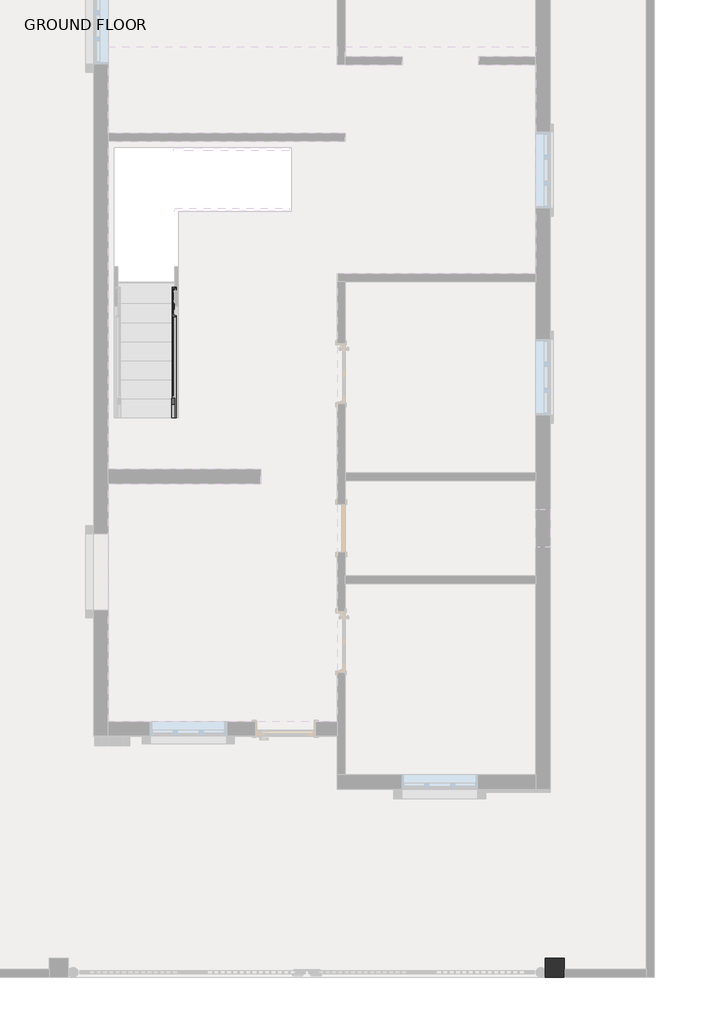
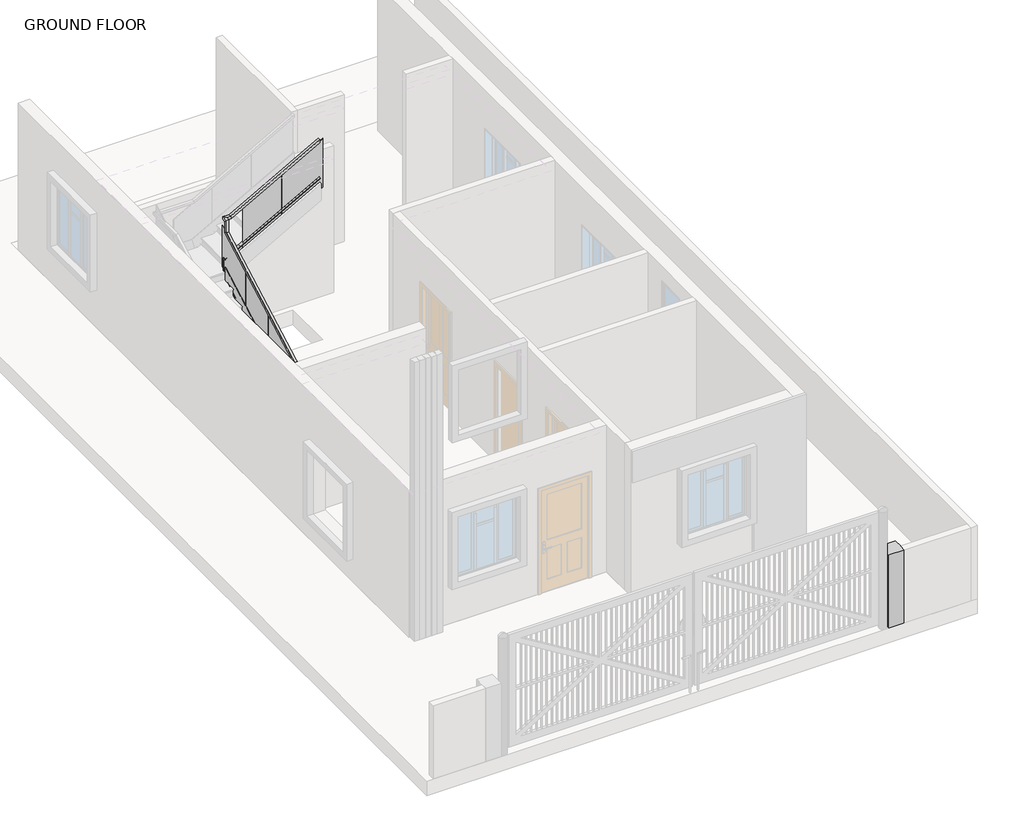
# One storey, part 2 of 4: 1 column, 1 railing.
"""IFC4 building model written with IfcOpenShell, lengths in millimetres."""

from ifc_helpers import new_model, si_unit, frame, origin, place, context, project, spatial, polyline, ellipse_curve, outline, extrude, faceted_brep, element, save
from ifc_brep_helpers import plane_surface, cylinder_surface, revolved_surface, advanced_brep

model = new_model("IFC4")

# Units and contexts
model_context = context("Model", 3, world=origin())
ifc_project = project(units=[si_unit("LENGTHUNIT", "METRE", prefix="MILLI")], contexts=[model_context])

# Site, building, storey
site = spatial("IfcSite", under=ifc_project)
building = spatial("IfcBuilding", under=site)
storey = spatial("IfcBuildingStorey", under=building, Name="GROUND FLOOR", Elevation=304.8)

# Column
placement = place(None, origin())
element("IfcColumn", 1, ObjectType="Rectangular Column : 1'X 1'", at=placement, inside=storey, context=model_context, shape_type="Brep", body=[
    faceted_brep([(-2180.0610805, -9269.5210084, 304.8), (-2180.0610805, -9447.3210084, 304.8), (-2180.0610805, -9574.3210084, 304.8), (-2484.8610805, -9574.3210084, 304.8), (-2484.8610805, -9269.5210084, 304.8), (-2180.0610805, -9269.5210084, 1828.8), (-2180.0610805, -9447.3210084, 1828.8), (-2180.0610805, -9574.3210084, 1828.8), (-2484.8610805, -9574.3210084, 1828.8), (-2484.8610805, -9269.5210084, 1828.8)], [[[0, 1, 2, 3, 4]], [[5, 6, 7, 2, 1, 0]], [[7, 8, 3, 2]], [[8, 9, 4, 3]], [[9, 5, 0, 4]], [[5, 9, 8, 7, 6]]]),
])

# Railing
element("IfcRailing", 2, ObjectType="GLASS PANEL RAILING", at=placement, inside=storey, context=model_context, shape_type="SolidModel", body=[
    faceted_brep([(-8451.9607439, -642.5827462, 1388.5333333), (-8451.9607439, -642.5827462, 1330.420221), (-8401.1607439, -642.5827462, 1330.420221), (-8401.1607439, -642.5827462, 1388.5333333), (-8451.9607439, 2634.0172538, 3208.8666667), (-8451.9607439, 2684.8172538, 3178.9757765), (-8401.1607439, 2684.8172538, 3178.9757765), (-8401.1607439, 2634.0172538, 3208.8666667), (-8451.9607439, 2634.0172538, 3462.8666667), (-8451.9607439, 2684.8172538, 3412.0666667), (-8401.1607439, 2684.8172538, 3412.0666667), (-8401.1607439, 2634.0172538, 3462.8666667), (-8451.9607439, 2761.0172538, 3462.8666667), (-8451.9607439, 2761.0172538, 3412.0666667), (-8401.1607439, 2710.2172538, 3412.0666667), (-8401.1607439, 2710.2172538, 3462.8666667), (-8324.9607439, 2761.0172538, 3462.8666667), (-8311.7971417, 2761.0172538, 3412.0666667), (-8311.7971417, 2710.2172538, 3412.0666667), (-8324.9607439, 2710.2172538, 3462.8666667), (-6572.3607439, 2761.0172538, 4436.5333333), (-6572.3607439, 2710.2172538, 4436.5333333), (-6572.3607439, 2710.2172538, 4378.420221), (-6572.3607439, 2761.0172538, 4378.420221)], [[[0, 1, 2, 3]], [[1, 0, 4, 5]], [[2, 1, 5, 6]], [[3, 2, 6, 7]], [[0, 3, 7, 4]], [[5, 4, 8, 9]], [[6, 5, 9, 10]], [[7, 6, 10, 11]], [[4, 7, 11, 8]], [[9, 8, 12, 13]], [[10, 9, 13, 14]], [[11, 10, 14, 15]], [[8, 11, 15, 12]], [[13, 12, 16, 17]], [[14, 13, 17, 18]], [[15, 14, 18, 19]], [[12, 15, 19, 16]], [[20, 21, 22, 23]], [[17, 16, 20, 23]], [[18, 17, 23, 22]], [[19, 18, 22, 21]], [[16, 19, 21, 20]]]),
    advanced_brep(
    [(-8441.4451439, -642.5827462, 604.8878361), (-8441.4451439, -642.5827462, 343.3788305), (-8378.1991439, -642.5827462, 343.3788305), (-8378.1991439, -642.5827462, 344.957123), (-8382.5819531, -642.5827462, 350.8756626), (-8406.2026439, -642.5827462, 355.3791882), (-8425.4405255, -642.5827462, 359.0470866), (-8434.2061439, -642.5827462, 370.8841659), (-8434.2061439, -642.5827462, 577.3825008), (-8425.4405255, -642.5827462, 589.2195801), (-8406.2026439, -642.5827462, 592.8874784), (-8382.5819531, -642.5827462, 597.391004), (-8378.1991439, -642.5827462, 603.3095437), (-8378.1991439, -642.5827462, 604.8878361), (-8441.4451439, 2687.2556538, 2454.7980583), (-8378.1991439, 2687.2556538, 2454.7980583), (-8378.1991439, 2687.2556538, 2453.2197659), (-8382.5819531, 2687.2556538, 2447.3012262), (-8406.2026439, 2687.2556538, 2442.7977006), (-8425.4405255, 2687.2556538, 2439.1298023), (-8434.2061439, 2687.2556538, 2427.292723), (-8434.2061439, 2687.2556538, 2220.7943881), (-8425.4405255, 2687.2556538, 2208.9573088), (-8406.2026439, 2687.2556538, 2205.2894105), (-8382.5819531, 2687.2556538, 2200.7858849), (-8378.1991439, 2687.2556538, 2194.8673452), (-8378.1991439, 2687.2556538, 2193.2890528), (-8441.4451439, 2687.2556538, 2193.2890528)],
    [
        (0, 1),
        (1, 2),
        (2, 3),
        (3, 4, ellipse_curve(frame((-8383.4442439, -642.5827462, 344.957123), z_axis=(0.0, -1.0, 0.0), x_axis=(0.0, 0.0, -1.0)), 6.0001789, 5.2451)),
        (4, 5),
        (5, 6),
        (6, 7, ellipse_curve(frame((-8423.7159439, -642.5827462, 370.8841659), z_axis=(0.0, 1.0, 0.0), x_axis=(0.0, 0.0, 1.0)), 12.0003577, 10.4902)),
        (7, 8),
        (8, 9, ellipse_curve(frame((-8423.7159439, -642.5827462, 577.3825008), z_axis=(0.0, 1.0, 0.0), x_axis=(0.0, 0.0, 1.0)), 12.0003577, 10.4902)),
        (9, 10),
        (10, 11),
        (11, 12, ellipse_curve(frame((-8383.4442439, -642.5827462, 603.3095437), z_axis=(0.0, -1.0, 0.0), x_axis=(0.0, 0.0, -1.0)), 6.0001789, 5.2451)),
        (12, 13),
        (13, 0),
        (14, 15),
        (15, 16),
        (16, 17, ellipse_curve(frame((-8383.4442439, 2687.2556538, 2453.2197659), z_axis=(0.0, 1.0, 0.0), x_axis=(0.0, 0.0, -1.0)), 6.0001789, 5.2451)),
        (17, 18),
        (18, 19),
        (19, 20, ellipse_curve(frame((-8423.7159439, 2687.2556538, 2427.292723), z_axis=(0.0, -1.0, 0.0), x_axis=(0.0, 0.0, 1.0)), 12.0003577, 10.4902)),
        (20, 21),
        (21, 22, ellipse_curve(frame((-8423.7159439, 2687.2556538, 2220.7943881), z_axis=(0.0, -1.0, 0.0), x_axis=(0.0, 0.0, 1.0)), 12.0003577, 10.4902)),
        (22, 23),
        (23, 24),
        (24, 25, ellipse_curve(frame((-8383.4442439, 2687.2556538, 2194.8673452), z_axis=(0.0, 1.0, 0.0), x_axis=(0.0, 0.0, -1.0)), 6.0001789, 5.2451)),
        (25, 26),
        (26, 27),
        (27, 14),
        (0, 14),
        (27, 1),
        (26, 2),
        (25, 3),
        (24, 4),
        (23, 5),
        (22, 6),
        (21, 7),
        (20, 8),
        (19, 9),
        (18, 10),
        (17, 11),
        (16, 12),
        (15, 13),
    ],
    [
        plane_surface(frame((-8426.5607439, -642.5827462, 474.1333333), z_axis=(0.0, -1.0, 0.0), x_axis=(0.0, 0.0, 1.0))),
        plane_surface(frame((-8426.5607439, 2687.2556538, 2324.0435556), z_axis=(0.0, 1.0, 0.0), x_axis=(0.0, 0.0, 1.0))),
        plane_surface(frame((-8441.4451439, -642.5827462, 604.8878361), z_axis=(-1.0, 0.0, 0.0), x_axis=(0.0, 0.8741572761215384, 0.48564293117863094))),
        plane_surface(frame((-8441.4451439, -642.5827462, 343.3788305), z_axis=(0.0, 0.48564293117863094, -0.8741572761215385), x_axis=(0.0, 0.8741572761215385, 0.48564293117863094))),
        plane_surface(frame((-8378.1991439, -642.5827462, 343.3788305), z_axis=(1.0, 0.0, 0.0), x_axis=(0.0, 0.8741572761215384, 0.48564293117863094))),
        cylinder_surface(frame((-8383.4442439, -587.7437889, 375.4232103), z_axis=(0.0, -0.8741572761215384, -0.48564293117863094), x_axis=(1.0, 0.0, 0.0)), 5.2451),
        plane_surface(frame((-8382.5819531, -642.5827462, 350.8756626), z_axis=(0.16439930721687715, -0.4790352105728132, 0.8622633790310658), x_axis=(0.0, 0.8741572761215384, 0.48564293117863094))),
        plane_surface(frame((-8406.2026439, -642.5827462, 355.3791882), z_axis=(0.16439930721687612, -0.4790352105728133, 0.862263379031066), x_axis=(0.0, 0.8741572761215384, 0.48564293117863094))),
        revolved_surface(polyline([(-8413.2257439, 2692.350145300002, 2223.6246610999956), (-8413.2257439, -647.6772376433962, 368.0538927981132)]), (-8423.7159439, -598.7505524, 395.2353846), (0.0, 0.8741572761215384, 0.48564293117863094)),
        plane_surface(frame((-8434.2061439, -642.5827462, 370.8841659), z_axis=(1.0, 0.0, 0.0), x_axis=(0.0, 0.8741572761215385, 0.4856429311786309))),
        revolved_surface(polyline([(-8413.2257439, 2692.3501452575492, 2430.1229960764103), (-8413.2257439, -647.677237685849, 574.5522277745283)]), (-8423.7159439, -686.4149399, 553.0312821), (0.0, 0.8741572761215384, 0.48564293117863094)),
        plane_surface(frame((-8425.4405255, -642.5827462, 589.2195801), z_axis=(0.16439930721687224, 0.4790352105728131, -0.8622633790310668), x_axis=(0.0, 0.8741572761215384, 0.48564293117863094))),
        plane_surface(frame((-8406.2026439, -642.5827462, 592.8874784), z_axis=(0.16439930721687154, 0.4790352105728131, -0.8622633790310668), x_axis=(0.0, 0.8741572761215384, 0.48564293117863094))),
        cylinder_surface(frame((-8383.4442439, -697.4217034, 572.8434563), z_axis=(0.0, -0.8741572761215384, -0.48564293117863094), x_axis=(1.0, 0.0, 0.0)), 5.2451),
        plane_surface(frame((-8378.1991439, -642.5827462, 603.3095437), z_axis=(1.0000000000000002, 0.0, 0.0), x_axis=(0.0, 0.8741572761215385, 0.48564293117863094))),
        plane_surface(frame((-8378.1991439, -642.5827462, 604.8878361), z_axis=(0.0, -0.48564293117863094, 0.8741572761215384), x_axis=(0.0, 0.8741572761215384, 0.48564293117863094))),
    ],
    [
        (0, [[1, 2, 3, 4, 5, 6, 7, 8, 9, 10, 11, 12, 13, 14]]),
        (1, [[15, 16, 17, 18, 19, 20, 21, 22, 23, 24, 25, 26, 27, 28]]),
        (2, [[-1, 29, -28, 30]]),
        (3, [[-2, -30, -27, 31]]),
        (4, [[-3, -31, -26, 32]]),
        (5, [[-4, -32, -25, 33]]),
        (6, [[-5, -33, -24, 34]]),
        (7, [[-6, -34, -23, 35]]),
        (8, [[-7, -35, -22, 36]]),
        (9, [[-8, -36, -21, 37]]),
        (10, [[-9, -37, -20, 38]]),
        (11, [[-10, -38, -19, 39]]),
        (12, [[-11, -39, -18, 40]]),
        (13, [[-12, -40, -17, 41]]),
        (14, [[-13, -41, -16, 42]]),
        (15, [[-14, -42, -15, -29]]),
    ],
),
    advanced_brep(
    [(-8441.4451439, 2750.5016538, 2614.5076139), (-8441.4451439, 2750.5016538, 2352.9986083), (-8441.4451439, 2687.2556538, 2352.9986083), (-8441.4451439, 2687.2556538, 2354.5769008), (-8441.4451439, 2691.638463, 2360.4954404), (-8441.4451439, 2715.2591538, 2364.998966), (-8441.4451439, 2734.4970355, 2368.6668644), (-8441.4451439, 2743.2626538, 2380.5039436), (-8441.4451439, 2743.2626538, 2587.0022786), (-8441.4451439, 2734.4970355, 2598.8393579), (-8441.4451439, 2715.2591538, 2602.5072562), (-8441.4451439, 2691.638463, 2607.0107818), (-8441.4451439, 2687.2556538, 2612.9293214), (-8441.4451439, 2687.2556538, 2614.5076139), (-6572.3607439, 2750.5016538, 3652.8878361), (-6572.3607439, 2687.2556538, 3652.8878361), (-6572.3607439, 2687.2556538, 3651.3095437), (-6572.3607439, 2691.638463, 3645.391004), (-6572.3607439, 2715.2591538, 3640.8874784), (-6572.3607439, 2734.4970355, 3637.2195801), (-6572.3607439, 2743.2626538, 3625.3825008), (-6572.3607439, 2743.2626538, 3418.8841659), (-6572.3607439, 2734.4970355, 3407.0470866), (-6572.3607439, 2715.2591538, 3403.3791882), (-6572.3607439, 2691.638463, 3398.8756626), (-6572.3607439, 2687.2556538, 3392.957123), (-6572.3607439, 2687.2556538, 3391.3788305), (-6572.3607439, 2750.5016538, 3391.3788305)],
    [
        (0, 1),
        (1, 2),
        (2, 3),
        (3, 4, ellipse_curve(frame((-8441.4451439, 2692.5007538, 2354.5769008), z_axis=(-1.0, 0.0, 0.0), x_axis=(0.0, 0.0, -1.0)), 6.0001789, 5.2451)),
        (4, 5),
        (5, 6),
        (6, 7, ellipse_curve(frame((-8441.4451439, 2732.7724538, 2380.5039436), z_axis=(1.0, 0.0, 0.0), x_axis=(0.0, 0.0, 1.0)), 12.0003577, 10.4902)),
        (7, 8),
        (8, 9, ellipse_curve(frame((-8441.4451439, 2732.7724538, 2587.0022786), z_axis=(1.0, 0.0, 0.0), x_axis=(0.0, 0.0, 1.0)), 12.0003577, 10.4902)),
        (9, 10),
        (10, 11),
        (11, 12, ellipse_curve(frame((-8441.4451439, 2692.5007538, 2612.9293214), z_axis=(-1.0, 0.0, 0.0), x_axis=(0.0, 0.0, -1.0)), 6.0001789, 5.2451)),
        (12, 13),
        (13, 0),
        (14, 15),
        (15, 16),
        (16, 17, ellipse_curve(frame((-6572.3607439, 2692.5007538, 3651.3095437), z_axis=(1.0, 0.0, 0.0), x_axis=(0.0, 0.0, -1.0)), 6.0001789, 5.2451)),
        (17, 18),
        (18, 19),
        (19, 20, ellipse_curve(frame((-6572.3607439, 2732.7724538, 3625.3825008), z_axis=(-1.0, 0.0, 0.0), x_axis=(0.0, 0.0, 1.0)), 12.0003577, 10.4902)),
        (20, 21),
        (21, 22, ellipse_curve(frame((-6572.3607439, 2732.7724538, 3418.8841659), z_axis=(-1.0, 0.0, 0.0), x_axis=(0.0, 0.0, 1.0)), 12.0003577, 10.4902)),
        (22, 23),
        (23, 24),
        (24, 25, ellipse_curve(frame((-6572.3607439, 2692.5007538, 3392.957123), z_axis=(1.0, 0.0, 0.0), x_axis=(0.0, 0.0, -1.0)), 6.0001789, 5.2451)),
        (25, 26),
        (26, 27),
        (27, 14),
        (0, 14),
        (27, 1),
        (26, 2),
        (25, 3),
        (24, 4),
        (23, 5),
        (22, 6),
        (21, 7),
        (20, 8),
        (19, 9),
        (18, 10),
        (17, 11),
        (16, 12),
        (15, 13),
    ],
    [
        plane_surface(frame((-8441.4451439, 2735.6172538, 2483.7531111), z_axis=(-1.0, 0.0, 0.0), x_axis=(0.0, 1.0, 0.0))),
        plane_surface(frame((-6572.3607439, 2735.6172538, 3522.1333333), z_axis=(1.0, 0.0, 0.0), x_axis=(0.0, 1.0, 0.0))),
        plane_surface(frame((-8441.4451439, 2750.5016538, 2614.5076139), z_axis=(0.0, 1.0, 0.0), x_axis=(0.8741572761215383, 0.0, 0.48564293117863133))),
        plane_surface(frame((-8441.4451439, 2750.5016538, 2352.9986083), z_axis=(0.4856429311786311, 0.0, -0.8741572761215384), x_axis=(0.8741572761215384, 0.0, 0.4856429311786311))),
        plane_surface(frame((-8441.4451439, 2687.2556538, 2352.9986083), z_axis=(0.0, -1.0, 0.0), x_axis=(0.8741572761215383, 0.0, 0.4856429311786312))),
        cylinder_surface(frame((-8386.6061867, 2692.5007538, 2385.0429881), z_axis=(-0.8741572761215383, 0.0, -0.48564293117863105), x_axis=(0.0, -1.0, 0.0)), 5.2451),
        plane_surface(frame((-8441.4451439, 2691.638463, 2360.4954404), z_axis=(-0.4790352105728135, -0.1643993072168764, 0.8622633790310658), x_axis=(0.8741572761215384, 0.0, 0.4856429311786311))),
        plane_surface(frame((-8441.4451439, 2715.2591538, 2364.998966), z_axis=(-0.47903521057281384, -0.1643993072168754, 0.8622633790310659), x_axis=(0.8741572761215383, 0.0, 0.48564293117863133))),
        revolved_surface(polyline([(-6567.266252423584, 2722.2822538, 3421.714438942451), (-8446.539635409434, 2722.2822538, 2377.6736706169813)]), (-8397.6129502, 2732.7724538, 2404.8551624), (0.8741572761215383, 0.0, 0.48564293117863105)),
        plane_surface(frame((-8441.4451439, 2743.2626538, 2380.5039436), z_axis=(0.0, -1.0, 0.0), x_axis=(0.8741572761215383, 0.0, 0.4856429311786312))),
        revolved_surface(polyline([(-6567.266252423584, 2722.2822538, 3628.21277384245), (-8446.539635366982, 2722.2822538, 2584.1720055405654)]), (-8485.2773377, 2732.7724538, 2562.6510598), (0.8741572761215383, 0.0, 0.48564293117863105)),
        plane_surface(frame((-8441.4451439, 2734.4970355, 2598.8393579), z_axis=(0.47903521057281295, -0.16439930721687304, -0.8622633790310668), x_axis=(0.8741572761215384, 0.0, 0.4856429311786311))),
        plane_surface(frame((-8441.4451439, 2715.2591538, 2602.5072562), z_axis=(0.47903521057281323, -0.16439930721687243, -0.8622633790310668), x_axis=(0.8741572761215383, 0.0, 0.48564293117863133))),
        cylinder_surface(frame((-8496.2841011, 2692.5007538, 2582.4632341), z_axis=(-0.8741572761215383, 0.0, -0.48564293117863105), x_axis=(0.0, -1.0, 0.0)), 5.2451),
        plane_surface(frame((-8441.4451439, 2687.2556538, 2612.9293214), z_axis=(0.0, -1.0, 0.0), x_axis=(0.8741572761215383, 0.0, 0.48564293117863133))),
        plane_surface(frame((-8441.4451439, 2687.2556538, 2614.5076139), z_axis=(-0.4856429311786311, 0.0, 0.8741572761215384), x_axis=(0.8741572761215384, 0.0, 0.4856429311786311))),
    ],
    [
        (0, [[1, 2, 3, 4, 5, 6, 7, 8, 9, 10, 11, 12, 13, 14]]),
        (1, [[15, 16, 17, 18, 19, 20, 21, 22, 23, 24, 25, 26, 27, 28]]),
        (2, [[-1, 29, -28, 30]]),
        (3, [[-2, -30, -27, 31]]),
        (4, [[-3, -31, -26, 32]]),
        (5, [[-4, -32, -25, 33]]),
        (6, [[-5, -33, -24, 34]]),
        (7, [[-6, -34, -23, 35]]),
        (8, [[-7, -35, -22, 36]]),
        (9, [[-8, -36, -21, 37]]),
        (10, [[-9, -37, -20, 38]]),
        (11, [[-10, -38, -19, 39]]),
        (12, [[-11, -39, -18, 40]]),
        (13, [[-12, -40, -17, 41]]),
        (14, [[-13, -41, -16, 42]]),
        (15, [[-14, -42, -15, -29]]),
    ],
),
    advanced_brep(
    [(-8441.4451439, -642.5827462, 604.8878361), (-8441.4451439, -642.5827462, 343.3788305), (-8378.1991439, -642.5827462, 343.3788305), (-8378.1991439, -642.5827462, 344.957123), (-8382.5819531, -642.5827462, 350.8756626), (-8406.2026439, -642.5827462, 355.3791882), (-8425.4405255, -642.5827462, 359.0470866), (-8434.2061439, -642.5827462, 370.8841659), (-8434.2061439, -642.5827462, 577.3825008), (-8425.4405255, -642.5827462, 589.2195801), (-8406.2026439, -642.5827462, 592.8874784), (-8382.5819531, -642.5827462, 597.391004), (-8378.1991439, -642.5827462, 603.3095437), (-8378.1991439, -642.5827462, 604.8878361), (-8441.4451439, 2687.2556538, 2454.7980583), (-8378.1991439, 2687.2556538, 2454.7980583), (-8378.1991439, 2687.2556538, 2453.2197659), (-8382.5819531, 2687.2556538, 2447.3012262), (-8406.2026439, 2687.2556538, 2442.7977006), (-8425.4405255, 2687.2556538, 2439.1298023), (-8434.2061439, 2687.2556538, 2427.292723), (-8434.2061439, 2687.2556538, 2220.7943881), (-8425.4405255, 2687.2556538, 2208.9573088), (-8406.2026439, 2687.2556538, 2205.2894105), (-8382.5819531, 2687.2556538, 2200.7858849), (-8378.1991439, 2687.2556538, 2194.8673452), (-8378.1991439, 2687.2556538, 2193.2890528), (-8441.4451439, 2687.2556538, 2193.2890528)],
    [
        (0, 1),
        (1, 2),
        (2, 3),
        (3, 4, ellipse_curve(frame((-8383.4442439, -642.5827462, 344.957123), z_axis=(0.0, -1.0, 0.0), x_axis=(0.0, 0.0, -1.0)), 6.0001789, 5.2451)),
        (4, 5),
        (5, 6),
        (6, 7, ellipse_curve(frame((-8423.7159439, -642.5827462, 370.8841659), z_axis=(0.0, 1.0, 0.0), x_axis=(0.0, 0.0, 1.0)), 12.0003577, 10.4902)),
        (7, 8),
        (8, 9, ellipse_curve(frame((-8423.7159439, -642.5827462, 577.3825008), z_axis=(0.0, 1.0, 0.0), x_axis=(0.0, 0.0, 1.0)), 12.0003577, 10.4902)),
        (9, 10),
        (10, 11),
        (11, 12, ellipse_curve(frame((-8383.4442439, -642.5827462, 603.3095437), z_axis=(0.0, -1.0, 0.0), x_axis=(0.0, 0.0, -1.0)), 6.0001789, 5.2451)),
        (12, 13),
        (13, 0),
        (14, 15),
        (15, 16),
        (16, 17, ellipse_curve(frame((-8383.4442439, 2687.2556538, 2453.2197659), z_axis=(0.0, 1.0, 0.0), x_axis=(0.0, 0.0, -1.0)), 6.0001789, 5.2451)),
        (17, 18),
        (18, 19),
        (19, 20, ellipse_curve(frame((-8423.7159439, 2687.2556538, 2427.292723), z_axis=(0.0, -1.0, 0.0), x_axis=(0.0, 0.0, 1.0)), 12.0003577, 10.4902)),
        (20, 21),
        (21, 22, ellipse_curve(frame((-8423.7159439, 2687.2556538, 2220.7943881), z_axis=(0.0, -1.0, 0.0), x_axis=(0.0, 0.0, 1.0)), 12.0003577, 10.4902)),
        (22, 23),
        (23, 24),
        (24, 25, ellipse_curve(frame((-8383.4442439, 2687.2556538, 2194.8673452), z_axis=(0.0, 1.0, 0.0), x_axis=(0.0, 0.0, -1.0)), 6.0001789, 5.2451)),
        (25, 26),
        (26, 27),
        (27, 14),
        (0, 14),
        (27, 1),
        (26, 2),
        (25, 3),
        (24, 4),
        (23, 5),
        (22, 6),
        (21, 7),
        (20, 8),
        (19, 9),
        (18, 10),
        (17, 11),
        (16, 12),
        (15, 13),
    ],
    [
        plane_surface(frame((-8426.5607439, -642.5827462, 474.1333333), z_axis=(0.0, -1.0, 0.0), x_axis=(0.0, 0.0, 1.0))),
        plane_surface(frame((-8426.5607439, 2687.2556538, 2324.0435556), z_axis=(0.0, 1.0, 0.0), x_axis=(0.0, 0.0, 1.0))),
        plane_surface(frame((-8441.4451439, -642.5827462, 604.8878361), z_axis=(-1.0, 0.0, 0.0), x_axis=(0.0, 0.8741572761215384, 0.48564293117863094))),
        plane_surface(frame((-8441.4451439, -642.5827462, 343.3788305), z_axis=(0.0, 0.48564293117863094, -0.8741572761215385), x_axis=(0.0, 0.8741572761215385, 0.48564293117863094))),
        plane_surface(frame((-8378.1991439, -642.5827462, 343.3788305), z_axis=(1.0, 0.0, 0.0), x_axis=(0.0, 0.8741572761215384, 0.48564293117863094))),
        cylinder_surface(frame((-8383.4442439, -587.7437889, 375.4232103), z_axis=(0.0, -0.8741572761215384, -0.48564293117863094), x_axis=(1.0, 0.0, 0.0)), 5.2451),
        plane_surface(frame((-8382.5819531, -642.5827462, 350.8756626), z_axis=(0.16439930721687715, -0.4790352105728132, 0.8622633790310658), x_axis=(0.0, 0.8741572761215384, 0.48564293117863094))),
        plane_surface(frame((-8406.2026439, -642.5827462, 355.3791882), z_axis=(0.16439930721687612, -0.4790352105728133, 0.862263379031066), x_axis=(0.0, 0.8741572761215384, 0.48564293117863094))),
        revolved_surface(polyline([(-8413.2257439, 2692.350145300002, 2223.6246610999956), (-8413.2257439, -647.6772376433962, 368.0538927981132)]), (-8423.7159439, -598.7505524, 395.2353846), (0.0, 0.8741572761215384, 0.48564293117863094)),
        plane_surface(frame((-8434.2061439, -642.5827462, 370.8841659), z_axis=(1.0, 0.0, 0.0), x_axis=(0.0, 0.8741572761215385, 0.4856429311786309))),
        revolved_surface(polyline([(-8413.2257439, 2692.3501452575492, 2430.1229960764103), (-8413.2257439, -647.677237685849, 574.5522277745283)]), (-8423.7159439, -686.4149399, 553.0312821), (0.0, 0.8741572761215384, 0.48564293117863094)),
        plane_surface(frame((-8425.4405255, -642.5827462, 589.2195801), z_axis=(0.16439930721687224, 0.4790352105728131, -0.8622633790310668), x_axis=(0.0, 0.8741572761215384, 0.48564293117863094))),
        plane_surface(frame((-8406.2026439, -642.5827462, 592.8874784), z_axis=(0.16439930721687154, 0.4790352105728131, -0.8622633790310668), x_axis=(0.0, 0.8741572761215384, 0.48564293117863094))),
        cylinder_surface(frame((-8383.4442439, -697.4217034, 572.8434563), z_axis=(0.0, -0.8741572761215384, -0.48564293117863094), x_axis=(1.0, 0.0, 0.0)), 5.2451),
        plane_surface(frame((-8378.1991439, -642.5827462, 603.3095437), z_axis=(1.0000000000000002, 0.0, 0.0), x_axis=(0.0, 0.8741572761215385, 0.48564293117863094))),
        plane_surface(frame((-8378.1991439, -642.5827462, 604.8878361), z_axis=(0.0, -0.48564293117863094, 0.8741572761215384), x_axis=(0.0, 0.8741572761215384, 0.48564293117863094))),
    ],
    [
        (0, [[1, 2, 3, 4, 5, 6, 7, 8, 9, 10, 11, 12, 13, 14]]),
        (1, [[15, 16, 17, 18, 19, 20, 21, 22, 23, 24, 25, 26, 27, 28]]),
        (2, [[-1, 29, -28, 30]]),
        (3, [[-2, -30, -27, 31]]),
        (4, [[-3, -31, -26, 32]]),
        (5, [[-4, -32, -25, 33]]),
        (6, [[-5, -33, -24, 34]]),
        (7, [[-6, -34, -23, 35]]),
        (8, [[-7, -35, -22, 36]]),
        (9, [[-8, -36, -21, 37]]),
        (10, [[-9, -37, -20, 38]]),
        (11, [[-10, -38, -19, 39]]),
        (12, [[-11, -39, -18, 40]]),
        (13, [[-12, -40, -17, 41]]),
        (14, [[-13, -41, -16, 42]]),
        (15, [[-14, -42, -15, -29]]),
    ],
),
    advanced_brep(
    [(-8441.4451439, 2750.5016538, 2614.5076139), (-8441.4451439, 2750.5016538, 2352.9986083), (-8441.4451439, 2687.2556538, 2352.9986083), (-8441.4451439, 2687.2556538, 2354.5769008), (-8441.4451439, 2691.638463, 2360.4954404), (-8441.4451439, 2715.2591538, 2364.998966), (-8441.4451439, 2734.4970355, 2368.6668644), (-8441.4451439, 2743.2626538, 2380.5039436), (-8441.4451439, 2743.2626538, 2587.0022786), (-8441.4451439, 2734.4970355, 2598.8393579), (-8441.4451439, 2715.2591538, 2602.5072562), (-8441.4451439, 2691.638463, 2607.0107818), (-8441.4451439, 2687.2556538, 2612.9293214), (-8441.4451439, 2687.2556538, 2614.5076139), (-6572.3607439, 2750.5016538, 3652.8878361), (-6572.3607439, 2687.2556538, 3652.8878361), (-6572.3607439, 2687.2556538, 3651.3095437), (-6572.3607439, 2691.638463, 3645.391004), (-6572.3607439, 2715.2591538, 3640.8874784), (-6572.3607439, 2734.4970355, 3637.2195801), (-6572.3607439, 2743.2626538, 3625.3825008), (-6572.3607439, 2743.2626538, 3418.8841659), (-6572.3607439, 2734.4970355, 3407.0470866), (-6572.3607439, 2715.2591538, 3403.3791882), (-6572.3607439, 2691.638463, 3398.8756626), (-6572.3607439, 2687.2556538, 3392.957123), (-6572.3607439, 2687.2556538, 3391.3788305), (-6572.3607439, 2750.5016538, 3391.3788305)],
    [
        (0, 1),
        (1, 2),
        (2, 3),
        (3, 4, ellipse_curve(frame((-8441.4451439, 2692.5007538, 2354.5769008), z_axis=(-1.0, 0.0, 0.0), x_axis=(0.0, 0.0, -1.0)), 6.0001789, 5.2451)),
        (4, 5),
        (5, 6),
        (6, 7, ellipse_curve(frame((-8441.4451439, 2732.7724538, 2380.5039436), z_axis=(1.0, 0.0, 0.0), x_axis=(0.0, 0.0, 1.0)), 12.0003577, 10.4902)),
        (7, 8),
        (8, 9, ellipse_curve(frame((-8441.4451439, 2732.7724538, 2587.0022786), z_axis=(1.0, 0.0, 0.0), x_axis=(0.0, 0.0, 1.0)), 12.0003577, 10.4902)),
        (9, 10),
        (10, 11),
        (11, 12, ellipse_curve(frame((-8441.4451439, 2692.5007538, 2612.9293214), z_axis=(-1.0, 0.0, 0.0), x_axis=(0.0, 0.0, -1.0)), 6.0001789, 5.2451)),
        (12, 13),
        (13, 0),
        (14, 15),
        (15, 16),
        (16, 17, ellipse_curve(frame((-6572.3607439, 2692.5007538, 3651.3095437), z_axis=(1.0, 0.0, 0.0), x_axis=(0.0, 0.0, -1.0)), 6.0001789, 5.2451)),
        (17, 18),
        (18, 19),
        (19, 20, ellipse_curve(frame((-6572.3607439, 2732.7724538, 3625.3825008), z_axis=(-1.0, 0.0, 0.0), x_axis=(0.0, 0.0, 1.0)), 12.0003577, 10.4902)),
        (20, 21),
        (21, 22, ellipse_curve(frame((-6572.3607439, 2732.7724538, 3418.8841659), z_axis=(-1.0, 0.0, 0.0), x_axis=(0.0, 0.0, 1.0)), 12.0003577, 10.4902)),
        (22, 23),
        (23, 24),
        (24, 25, ellipse_curve(frame((-6572.3607439, 2692.5007538, 3392.957123), z_axis=(1.0, 0.0, 0.0), x_axis=(0.0, 0.0, -1.0)), 6.0001789, 5.2451)),
        (25, 26),
        (26, 27),
        (27, 14),
        (0, 14),
        (27, 1),
        (26, 2),
        (25, 3),
        (24, 4),
        (23, 5),
        (22, 6),
        (21, 7),
        (20, 8),
        (19, 9),
        (18, 10),
        (17, 11),
        (16, 12),
        (15, 13),
    ],
    [
        plane_surface(frame((-8441.4451439, 2735.6172538, 2483.7531111), z_axis=(-1.0, 0.0, 0.0), x_axis=(0.0, 1.0, 0.0))),
        plane_surface(frame((-6572.3607439, 2735.6172538, 3522.1333333), z_axis=(1.0, 0.0, 0.0), x_axis=(0.0, 1.0, 0.0))),
        plane_surface(frame((-8441.4451439, 2750.5016538, 2614.5076139), z_axis=(0.0, 1.0, 0.0), x_axis=(0.8741572761215383, 0.0, 0.48564293117863133))),
        plane_surface(frame((-8441.4451439, 2750.5016538, 2352.9986083), z_axis=(0.4856429311786311, 0.0, -0.8741572761215384), x_axis=(0.8741572761215384, 0.0, 0.4856429311786311))),
        plane_surface(frame((-8441.4451439, 2687.2556538, 2352.9986083), z_axis=(0.0, -1.0, 0.0), x_axis=(0.8741572761215383, 0.0, 0.4856429311786312))),
        cylinder_surface(frame((-8386.6061867, 2692.5007538, 2385.0429881), z_axis=(-0.8741572761215383, 0.0, -0.48564293117863105), x_axis=(0.0, -1.0, 0.0)), 5.2451),
        plane_surface(frame((-8441.4451439, 2691.638463, 2360.4954404), z_axis=(-0.4790352105728135, -0.1643993072168764, 0.8622633790310658), x_axis=(0.8741572761215384, 0.0, 0.4856429311786311))),
        plane_surface(frame((-8441.4451439, 2715.2591538, 2364.998966), z_axis=(-0.47903521057281384, -0.1643993072168754, 0.8622633790310659), x_axis=(0.8741572761215383, 0.0, 0.48564293117863133))),
        revolved_surface(polyline([(-6567.266252423584, 2722.2822538, 3421.714438942451), (-8446.539635409434, 2722.2822538, 2377.6736706169813)]), (-8397.6129502, 2732.7724538, 2404.8551624), (0.8741572761215383, 0.0, 0.48564293117863105)),
        plane_surface(frame((-8441.4451439, 2743.2626538, 2380.5039436), z_axis=(0.0, -1.0, 0.0), x_axis=(0.8741572761215383, 0.0, 0.4856429311786312))),
        revolved_surface(polyline([(-6567.266252423584, 2722.2822538, 3628.21277384245), (-8446.539635366982, 2722.2822538, 2584.1720055405654)]), (-8485.2773377, 2732.7724538, 2562.6510598), (0.8741572761215383, 0.0, 0.48564293117863105)),
        plane_surface(frame((-8441.4451439, 2734.4970355, 2598.8393579), z_axis=(0.47903521057281295, -0.16439930721687304, -0.8622633790310668), x_axis=(0.8741572761215384, 0.0, 0.4856429311786311))),
        plane_surface(frame((-8441.4451439, 2715.2591538, 2602.5072562), z_axis=(0.47903521057281323, -0.16439930721687243, -0.8622633790310668), x_axis=(0.8741572761215383, 0.0, 0.48564293117863133))),
        cylinder_surface(frame((-8496.2841011, 2692.5007538, 2582.4632341), z_axis=(-0.8741572761215383, 0.0, -0.48564293117863105), x_axis=(0.0, -1.0, 0.0)), 5.2451),
        plane_surface(frame((-8441.4451439, 2687.2556538, 2612.9293214), z_axis=(0.0, -1.0, 0.0), x_axis=(0.8741572761215383, 0.0, 0.48564293117863133))),
        plane_surface(frame((-8441.4451439, 2687.2556538, 2614.5076139), z_axis=(-0.4856429311786311, 0.0, 0.8741572761215384), x_axis=(0.8741572761215384, 0.0, 0.4856429311786311))),
    ],
    [
        (0, [[1, 2, 3, 4, 5, 6, 7, 8, 9, 10, 11, 12, 13, 14]]),
        (1, [[15, 16, 17, 18, 19, 20, 21, 22, 23, 24, 25, 26, 27, 28]]),
        (2, [[-1, 29, -28, 30]]),
        (3, [[-2, -30, -27, 31]]),
        (4, [[-3, -31, -26, 32]]),
        (5, [[-4, -32, -25, 33]]),
        (6, [[-5, -33, -24, 34]]),
        (7, [[-6, -34, -23, 35]]),
        (8, [[-7, -35, -22, 36]]),
        (9, [[-8, -36, -21, 37]]),
        (10, [[-9, -37, -20, 38]]),
        (11, [[-10, -38, -19, 39]]),
        (12, [[-11, -39, -18, 40]]),
        (13, [[-12, -40, -17, 41]]),
        (14, [[-13, -41, -16, 42]]),
        (15, [[-14, -42, -15, -29]]),
    ],
),
    extrude(outline(polyline([(2957.6888889, -7308.9607439), (3409.2444444, -6496.1607439), (4420.7535543, -6496.1607439), (3969.1979988, -7308.9607439), (2957.6888889, -7308.9607439)])), frame((0.0, 2735.8024108, 0.0), z_axis=(0.0, 1.0, 0.0), x_axis=(0.0, 0.0, 1.0)), (0.0, 0.0, 1.0), 6.35),
    extrude(outline(polyline([(2619.0222222, -8070.9607439), (3070.5777778, -7258.1607439), (3997.420221, -7258.1607439), (3545.8646654, -8070.9607439), (2619.0222222, -8070.9607439)])), frame((0.0, 2735.8024108, 0.0), z_axis=(0.0, 1.0, 0.0), x_axis=(0.0, 0.0, 1.0)), (0.0, 0.0, 1.0), 6.35),
    extrude(outline(polyline([(1999.0172538, 1941.6888889), (1999.0172538, 2797.9757765), (2811.8172538, 3249.5313321), (2811.8172538, 2393.2444444), (1999.0172538, 1941.6888889)])), frame((-8433.0959009, 0.0, 0.0), z_axis=(1.0, 0.0, 0.0), x_axis=(0.0, 1.0, 0.0)), (0.0, 0.0, 1.0), 6.35),
    extrude(outline(polyline([(1237.0172538, 1433.6888889), (1237.0172538, 2374.6424432), (2049.8172538, 2826.1979988), (2049.8172538, 1885.2444444), (1237.0172538, 1433.6888889)])), frame((-8433.0959009, 0.0, 0.0), z_axis=(1.0, 0.0, 0.0), x_axis=(0.0, 1.0, 0.0)), (0.0, 0.0, 1.0), 6.35),
    extrude(outline(polyline([(475.0172538, 1095.0222222), (475.0172538, 1951.3091099), (1287.8172538, 2402.8646654), (1287.8172538, 1546.5777778), (475.0172538, 1095.0222222)])), frame((-8433.0959009, 0.0, 0.0), z_axis=(1.0, 0.0, 0.0), x_axis=(0.0, 1.0, 0.0)), (0.0, 0.0, 1.0), 6.35),
    extrude(outline(polyline([(-286.9827462, 587.0222222), (-286.9827462, 1527.9757765), (525.8172538, 1979.5313321), (525.8172538, 1038.5777778), (-286.9827462, 587.0222222)])), frame((-8433.0959009, 0.0, 0.0), z_axis=(1.0, 0.0, 0.0), x_axis=(0.0, 1.0, 0.0)), (0.0, 0.0, 1.0), 6.35),
])

save(model, "model.ifc")

# Revit data of these elements
# Type "Rectangular Column : 1'X 1'"
#   Assembly Code = "B1010200"
#   Depth = 1' - 0"
#   Offset Base = 0' - 0"
#   Offset Top = 0' - 0"
#   Width = 1' - 0"
# Type "GLASS PANEL RAILING"
#   Assembly Code = "C2010400"
#   built-in parameter 1008612 = 0.0416667 (stored number, unit not read)
#   built-in parameter 1008611 = 0.0416667 (stored number, unit not read)
#   built-in parameter 1008609 = 0.333333 (stored number, unit not read)
#   built-in parameter 1008604 = 0.166667 (stored number, unit not read)
#   built-in parameter 1008603 = 0.166667 (stored number, unit not read)
#   Railing Height = 3' - 0"
#   built-in parameter 1008630 = 2
#   built-in parameter 1008610 = 2
#   built-in parameter 1008618 = Baluster - Square : 3/4"
# Element 1 (IfcColumn, "Rectangular Column : 1'X 1'")
#   Phase Created = New Construction
# Element 2 (IfcRailing, "GLASS PANEL RAILING")
#   Phase Created = New Construction
#   Materials on its faces: "BLACK", "Glass"
# Materials
#   "BLACK": class "Generic", colour RGB 120 120 120, transparency 0, Cost = 0
#   "Glass": class "Glass", colour RGB 0 128 192, transparency 0.75, Description = "Soda Lime Glass", Cost = 0
